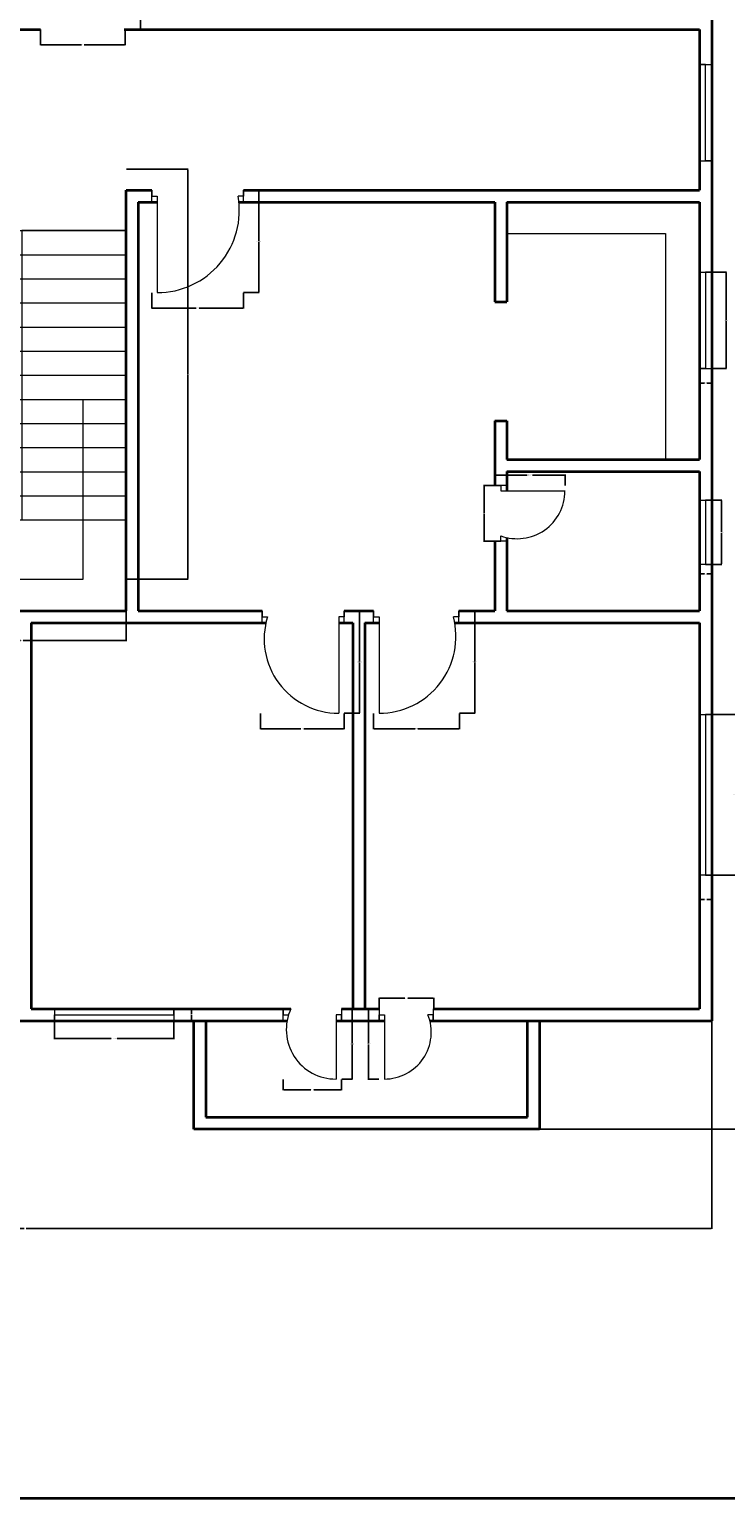
# Model space of a CAD drawing. Units: inches. Extents: x 1944 to 3454, y 1352 to 3055.
# Tile 11 of 17: x 2903 to 3163, y 1352 to 1900. Entities that reach past the tile are written whole.
import ezdxf

# ---------------------------------------------------------------- set-up
doc = ezdxf.new("R2010")
doc.units = ezdxf.units.IN
for name, color, linetype, lineweight in [('A-ANNO-DIMS', 2, 'Continuous', 18), ('A-ANNO-TTLB', 7, 'Continuous', 35), ('A-DOOR', 3, 'Continuous', 20), ('A-FLOR-CASE', 8, 'Continuous', 20), ('A-FLOR-STRS', 7, 'Continuous', 20), ('A-GLAZ', 4, 'Continuous', 18), ('A-WALL', 7, 'Continuous', 35)]:
    doc.layers.add(name, color=color, linetype=linetype, lineweight=lineweight)
doc.styles.get("Standard").update_dxf_attribs({"font": 'arial.ttf'})
doc.dimstyles.get("Standard").update_dxf_attribs({"dimtxt": 0.18, "dimasz": 0.18, "dimexe": 0.18, "dimexo": 0.0625, "dimgap": 0.09, "dimtad": 0, "dimtih": 1, "dimtoh": 1, "dimdec": 4, "dimzin": 0, "dimdsep": 46, "dimtxsty": 'Standard', "dimcen": 0.09, "dimadec": 0, "dimazin": 0, "dimtfac": 1, "dimtdec": 4, "dimtofl": 0, "dimtmove": 0, "dimatfit": 3, "dimfxl": 1, "dimtolj": 1, "dimtzin": 0, "dimarcsym": 0})

# ---------------------------------------------------------------- blocks, each defined once
blk = doc.blocks.new('DOOR-SWING-24IN-07')
for p, q in [((4.5, 20.75), (0, 20.75)), ((0, 20.75), (2.25, 20.75)), ((2.25, 20.75), (2.25, 18.75)), ((2.25, 18.75), (26.25, 18.75)), ((4.5, 0), (0, 0)), ((0, 0), (2.25, 0)), ((2.25, 0), (2.25, 2))]:
    blk.add_line(p, q)
blk.add_arc((8.4, 18.75), 17.84, 249.8228, 0)
blk = doc.blocks.new('DOOR-SWING-36IN-05')
for p, q in [((0, 33.75), (0, 38.25)), ((0, 38.25), (0, 36)), ((0, 36), (0, 36)), ((0, 36), (2, 36)), ((2, 36), (2, 0)), ((31.76, 36), (29.76, 36)), ((31.76, 33.75), (31.76, 38.25)), ((31.76, 38.25), (31.76, 36))]:
    blk.add_line(p, q)
blk.add_arc((2, 28.7), 28.7, 270, 14.7288)
blk = doc.blocks.new('DOOR-SWING-36IN-06')
for p, q in [((0, 33.75), (0, 38.25)), ((0, 38.25), (0, 36)), ((0, 36), (2, 36)), ((30.6, 36), (28.6, 36)), ((28.6, 36), (28.6, 0)), ((30.6, 33.75), (30.6, 38.25)), ((30.6, 38.25), (30.6, 36))]:
    blk.add_line(p, q)
blk.add_arc((28.6, 27.83), 27.83, 162.9212, 270)
blk = doc.blocks.new('DOOR-SWING-24IN-11')
for p, q in [((0, 21.75), (0, 26.25)), ((0, 26.25), (0, 24)), ((0, 24), (2, 24)), ((21.74, 24), (19.74, 24)), ((19.74, 24), (19.74, 0)), ((21.74, 26.25), (21.74, 21.75)), ((21.74, 21.75), (21.74, 24))]:
    blk.add_line(p, q)
blk.add_arc((19.54, 18.41), 18.41, 154.7737, 270.6503)
blk = doc.blocks.new('DOOR-SWING-24IN-12')
for p, q in [((0, 26.25), (0, 21.75)), ((0, 21.75), (0, 24)), ((0, 24), (2, 24)), ((2, 24), (2, 0)), ((20.24, 24), (18.24, 24)), ((20.24, 26.25), (20.24, 21.75)), ((20.24, 21.75), (20.24, 24))]:
    blk.add_line(p, q)
blk.add_arc((2.03, 17.47), 17.47, 269.8982, 21.9448)
blk = doc.blocks.new('DOOR-SWING-36IN-12')
for p, q in [((0, 33.75), (0, 38.25)), ((0, 38.25), (0, 36)), ((0, 36), (2, 36)), ((2, 36), (2, 0)), ((34.2, 36), (32.2, 36)), ((34.2, 33.75), (34.2, 38.25)), ((34.2, 38.25), (34.2, 36))]:
    blk.add_line(p, q)
blk.add_arc((2, 30.67), 30.67, 270, 10.0117)
blk = doc.blocks.new('WINDOW-PLAN-60.00IN-01')
for p, q in [((0, 60), (4.5, 60)), ((4.5, 60), (2.25, 60)), ((2.25, 60), (2.25, 0)), ((4.5, 0), (0, 0)), ((2.25, 0), (4.5, 0))]:
    blk.add_line(p, q)
blk = doc.blocks.new('WINDOW-PLAN-36.00IN-01')
for p, q in [((0, 36), (4.5, 36)), ((4.5, 36), (2.25, 36)), ((2.25, 36), (2.25, 0)), ((2.25, 0), (0, 0)), ((0, 0), (4.5, 0))]:
    blk.add_line(p, q)
blk = doc.blocks.new('WINDOW-PLAN-24.00IN-02')
for p, q in [((0, 24), (4.5, 24)), ((4.5, 24), (2.25, 24)), ((2.25, 24), (2.25, 0)), ((4.5, 0), (0, 0)), ((2.25, 0), (4.5, 0))]:
    blk.add_line(p, q)
blk = doc.blocks.new('WINDOW-PLAN-44.51IN-01')
for p, q in [((0, 4.5), (0, 0)), ((0, 0), (0, 2.25)), ((0, 2.25), (44.51, 2.25)), ((44.51, 2.25), (44.51, 4.5)), ((44.51, 4.5), (44.51, 0))]:
    blk.add_line(p, q)
blk = doc.blocks.new('STAIR-TWO-FLIGHT-01')
for p, q in [((18.12, 152.99), (18.12, 0)), ((0, 130.08), (78, 130.08)), ((78, 130.08), (39, 130.08)), ((39, 130.08), (39, 22.08)), ((0, 121.08), (78, 121.08)), ((0, 112.08), (78, 112.08)), ((0, 103.08), (78, 103.08)), ((0, 94.08), (78, 94.08)), ((0, 85.08), (78, 85.08)), ((0, 76.08), (78, 76.08)), ((0, 67.08), (78, 67.08)), ((61.93, 0), (61.93, 67.08)), ((0, 58.08), (78, 58.08)), ((0, 49.08), (78, 49.08)), ((0, 40.08), (78, 40.08)), ((0, 31.08), (78, 31.08)), ((0, 22.08), (78, 22.08)), ((18.12, 0), (61.93, 0))]:
    blk.add_line(p, q)
blk = doc.blocks.new('*D70')
at = {"layer": 'A-ANNO-DIMS', "color": 0, "lineweight": -2, "transparency": 16777216}
for p, q in [((3157.44, 1809.51), (3162.96, 1809.51)), ((3162.78, 1809.33), (3162.78, 1791.69)), ((3162.78, 1773.69), (3162.78, 1791.32)), ((3157.44, 1773.51), (3162.96, 1773.51))]:
    blk.add_line(p, q, dxfattribs=at)
at = {"layer": 'A-ANNO-DIMS', "color": 0, "transparency": 16777216}
for points in [[(3162.75, 1809.33), (3162.81, 1809.33), (3162.78, 1809.51)], [(3162.75, 1773.69), (3162.81, 1773.69), (3162.78, 1773.51)]]:
    blk.add_solid(points, dxfattribs=at)
at = {"layer": 'Defpoints', "color": 0, "transparency": 16777216}
for p in [(3157.38, 1809.51), (3162.78, 1809.51), (3157.38, 1773.51)]:
    blk.add_point(p, dxfattribs=at)
at = {"layer": 'A-ANNO-DIMS', "color": 0, "transparency": 16777216, "insert": (3162.78, 1791.51), "char_height": 0.18, "attachment_point": 5}
blk.add_mtext('\\A1;WINDOW 36 TYP.', dxfattribs=at)
blk = doc.blocks.new('*D71')
at = {"layer": 'A-ANNO-DIMS', "color": 0, "lineweight": -2, "transparency": 16777216}
for p, q in [((3152.88, 1773.44), (3152.88, 1767.93)), ((3157.38, 1773.44), (3157.38, 1767.93)), ((3153.06, 1768.11), (3154.67, 1768.11)), ((3157.2, 1768.11), (3155.58, 1768.11))]:
    blk.add_line(p, q, dxfattribs=at)
at = {"layer": 'A-ANNO-DIMS', "color": 0, "transparency": 16777216}
for points in [[(3153.06, 1768.14), (3153.06, 1768.08), (3152.88, 1768.11)], [(3157.2, 1768.14), (3157.2, 1768.08), (3157.38, 1768.11)]]:
    blk.add_solid(points, dxfattribs=at)
at = {"layer": 'Defpoints', "color": 0, "transparency": 16777216}
for p in [(3152.88, 1773.51), (3157.38, 1773.51), (3157.38, 1768.11)]:
    blk.add_point(p, dxfattribs=at)
at = {"layer": 'A-ANNO-DIMS', "color": 0, "transparency": 16777216, "insert": (3155.13, 1768.11), "char_height": 0.18, "attachment_point": 5}
blk.add_mtext('\\A1;5 TYP.', dxfattribs=at)
blk = doc.blocks.new('*D76')
at = {"layer": 'A-ANNO-DIMS', "color": 0, "lineweight": -2, "transparency": 16777216}
for p, q in [((3157.44, 1724.44), (3161.16, 1724.44)), ((3160.98, 1724.26), (3160.98, 1712.63)), ((3160.98, 1700.62), (3160.98, 1712.26)), ((3157.44, 1700.44), (3161.16, 1700.44))]:
    blk.add_line(p, q, dxfattribs=at)
at = {"layer": 'A-ANNO-DIMS', "color": 0, "transparency": 16777216}
for points in [[(3160.95, 1724.26), (3161.01, 1724.26), (3160.98, 1724.44)], [(3160.95, 1700.62), (3161.01, 1700.62), (3160.98, 1700.44)]]:
    blk.add_solid(points, dxfattribs=at)
at = {"layer": 'Defpoints', "color": 0, "transparency": 16777216}
for p in [(3157.38, 1724.44), (3160.98, 1724.44), (3157.38, 1700.44)]:
    blk.add_point(p, dxfattribs=at)
at = {"layer": 'A-ANNO-DIMS', "color": 0, "transparency": 16777216, "insert": (3160.98, 1712.44), "char_height": 0.18, "attachment_point": 5}
blk.add_mtext('\\A1;WINDOW 24 TYP.', dxfattribs=at)
blk = doc.blocks.new('*D77')
at = {"layer": 'A-ANNO-DIMS', "color": 0, "lineweight": -2, "transparency": 16777216}
for p, q in [((3152.88, 1700.38), (3152.88, 1696.66)), ((3157.38, 1700.38), (3157.38, 1696.66)), ((3153.06, 1696.84), (3154.67, 1696.84)), ((3157.2, 1696.84), (3155.58, 1696.84))]:
    blk.add_line(p, q, dxfattribs=at)
at = {"layer": 'A-ANNO-DIMS', "color": 0, "transparency": 16777216}
for points in [[(3153.06, 1696.87), (3153.06, 1696.81), (3152.88, 1696.84)], [(3157.2, 1696.87), (3157.2, 1696.81), (3157.38, 1696.84)]]:
    blk.add_solid(points, dxfattribs=at)
at = {"layer": 'Defpoints', "color": 0, "transparency": 16777216}
for p in [(3152.88, 1700.44), (3157.38, 1700.44), (3157.38, 1696.84)]:
    blk.add_point(p, dxfattribs=at)
at = {"layer": 'A-ANNO-DIMS', "color": 0, "transparency": 16777216, "insert": (3155.13, 1696.84), "char_height": 0.18, "attachment_point": 5}
blk.add_mtext('\\A1;5 TYP.', dxfattribs=at)
blk = doc.blocks.new('*D78')
at = {"layer": 'A-ANNO-DIMS', "color": 0, "lineweight": -2, "transparency": 16777216}
for p, q in [((3157.44, 1644.39), (3166.56, 1644.39)), ((3166.38, 1644.21), (3166.38, 1614.57)), ((3166.38, 1584.57), (3166.38, 1614.21)), ((3157.44, 1584.39), (3166.56, 1584.39))]:
    blk.add_line(p, q, dxfattribs=at)
at = {"layer": 'A-ANNO-DIMS', "color": 0, "transparency": 16777216}
for points in [[(3166.35, 1644.21), (3166.41, 1644.21), (3166.38, 1644.39)], [(3166.35, 1584.57), (3166.41, 1584.57), (3166.38, 1584.39)]]:
    blk.add_solid(points, dxfattribs=at)
at = {"layer": 'Defpoints', "color": 0, "transparency": 16777216}
for p in [(3157.38, 1644.39), (3166.38, 1644.39), (3157.38, 1584.39)]:
    blk.add_point(p, dxfattribs=at)
at = {"layer": 'A-ANNO-DIMS', "color": 0, "transparency": 16777216, "insert": (3166.38, 1614.39), "char_height": 0.18, "attachment_point": 5}
blk.add_mtext('\\A1;WINDOW 60 TYP.', dxfattribs=at)
blk = doc.blocks.new('*D79')
at = {"layer": 'A-ANNO-DIMS', "color": 0, "lineweight": -2, "transparency": 16777216}
for p, q in [((3152.88, 1584.33), (3152.88, 1575.21)), ((3157.38, 1584.33), (3157.38, 1575.21)), ((3153.06, 1575.39), (3154.67, 1575.39)), ((3157.2, 1575.39), (3155.58, 1575.39))]:
    blk.add_line(p, q, dxfattribs=at)
at = {"layer": 'A-ANNO-DIMS', "color": 0, "transparency": 16777216}
for points in [[(3153.06, 1575.42), (3153.06, 1575.36), (3152.88, 1575.39)], [(3157.2, 1575.42), (3157.2, 1575.36), (3157.38, 1575.39)]]:
    blk.add_solid(points, dxfattribs=at)
at = {"layer": 'Defpoints', "color": 0, "transparency": 16777216}
for p in [(3152.88, 1584.39), (3157.38, 1584.39), (3157.38, 1575.39)]:
    blk.add_point(p, dxfattribs=at)
at = {"layer": 'A-ANNO-DIMS', "color": 0, "transparency": 16777216, "insert": (3155.13, 1575.39), "char_height": 0.18, "attachment_point": 5}
blk.add_mtext('\\A1;5 TYP.', dxfattribs=at)
blk = doc.blocks.new('*D82')
at = {"layer": 'A-ANNO-DIMS', "color": 0, "lineweight": -2, "transparency": 16777216}
for p, q in [((2912.07, 1530.03), (2912.07, 1523.24)), ((2956.59, 1530.03), (2956.59, 1523.24)), ((2912.25, 1523.42), (2933.21, 1523.42)), ((2956.41, 1523.42), (2935.45, 1523.42))]:
    blk.add_line(p, q, dxfattribs=at)
at = {"layer": 'A-ANNO-DIMS', "color": 0, "transparency": 16777216}
for points in [[(2912.25, 1523.45), (2912.25, 1523.39), (2912.07, 1523.42)], [(2956.41, 1523.45), (2956.41, 1523.39), (2956.59, 1523.42)]]:
    blk.add_solid(points, dxfattribs=at)
at = {"layer": 'Defpoints', "color": 0, "transparency": 16777216}
for p in [(2912.07, 1530.1), (2956.59, 1530.1), (2956.59, 1523.42)]:
    blk.add_point(p, dxfattribs=at)
at = {"layer": 'A-ANNO-DIMS', "color": 0, "transparency": 16777216, "insert": (2934.33, 1523.42), "char_height": 0.18, "attachment_point": 5}
blk.add_mtext('\\A1;WINDOW 45 TYP.', dxfattribs=at)
blk = doc.blocks.new('*D83')
at = {"layer": 'A-ANNO-DIMS', "color": 0, "lineweight": -2, "transparency": 16777216}
for p, q in [((2956.65, 1534.6), (2963.44, 1534.6)), ((2956.65, 1530.1), (2963.44, 1530.1)), ((2963.26, 1534.42), (2963.26, 1532.53)), ((2963.26, 1530.28), (2963.26, 1532.16))]:
    blk.add_line(p, q, dxfattribs=at)
at = {"layer": 'A-ANNO-DIMS', "color": 0, "transparency": 16777216}
for points in [[(2963.23, 1534.42), (2963.29, 1534.42), (2963.26, 1534.6)], [(2963.23, 1530.28), (2963.29, 1530.28), (2963.26, 1530.1)]]:
    blk.add_solid(points, dxfattribs=at)
at = {"layer": 'Defpoints', "color": 0, "transparency": 16777216}
for p in [(2956.59, 1534.6), (2956.59, 1530.1), (2963.26, 1534.6)]:
    blk.add_point(p, dxfattribs=at)
at = {"layer": 'A-ANNO-DIMS', "color": 0, "transparency": 16777216, "insert": (2963.26, 1532.35), "char_height": 0.18, "attachment_point": 5}
blk.add_mtext('\\A1;5 TYP.', dxfattribs=at)
blk = doc.blocks.new('*D90')
at = {"layer": 'A-ANNO-DIMS', "color": 0, "lineweight": -2, "transparency": 16777216}
for p, q in [((2938.94, 1847.92), (2962, 1847.92)), ((2961.82, 1847.74), (2961.82, 1771.6)), ((2961.82, 1695.1), (2961.82, 1771.24)), ((2938.94, 1694.92), (2962, 1694.92))]:
    blk.add_line(p, q, dxfattribs=at)
at = {"layer": 'A-ANNO-DIMS', "color": 0, "transparency": 16777216}
for points in [[(2961.79, 1847.74), (2961.85, 1847.74), (2961.82, 1847.92)], [(2961.79, 1695.1), (2961.85, 1695.1), (2961.82, 1694.92)]]:
    blk.add_solid(points, dxfattribs=at)
at = {"layer": 'Defpoints', "color": 0, "transparency": 16777216}
for p in [(2938.88, 1847.92), (2961.82, 1847.92), (2938.88, 1694.92)]:
    blk.add_point(p, dxfattribs=at)
at = {"layer": 'A-ANNO-DIMS', "color": 0, "transparency": 16777216, "insert": (2961.82, 1771.42), "char_height": 0.18, "attachment_point": 5}
blk.add_mtext('\\A1;STAIR 153 TYP.', dxfattribs=at)
blk = doc.blocks.new('*D91')
at = {"layer": 'A-ANNO-DIMS', "color": 0, "lineweight": -2, "transparency": 16777216}
for p, q in [((2860.88, 1694.86), (2860.88, 1671.8)), ((2938.88, 1694.86), (2938.88, 1671.8)), ((2861.06, 1671.98), (2899.35, 1671.98)), ((2938.7, 1671.98), (2900.4, 1671.98))]:
    blk.add_line(p, q, dxfattribs=at)
at = {"layer": 'A-ANNO-DIMS', "color": 0, "transparency": 16777216}
for points in [[(2861.06, 1672.01), (2861.06, 1671.95), (2860.88, 1671.98)], [(2938.7, 1672.01), (2938.7, 1671.95), (2938.88, 1671.98)]]:
    blk.add_solid(points, dxfattribs=at)
at = {"layer": 'Defpoints', "color": 0, "transparency": 16777216}
for p in [(2860.88, 1694.92), (2938.88, 1694.92), (2938.88, 1671.98)]:
    blk.add_point(p, dxfattribs=at)
at = {"layer": 'A-ANNO-DIMS', "color": 0, "transparency": 16777216, "insert": (2899.88, 1671.98), "char_height": 0.18, "attachment_point": 5}
blk.add_mtext('\\A1;78 TYP.', dxfattribs=at)
blk = doc.blocks.new('*D100')
at = {"layer": 'A-ANNO-DIMS', "color": 0, "lineweight": -2, "transparency": 16777216}
for p, q in [((3063.29, 1683.1), (3069.15, 1683.1)), ((3068.97, 1682.92), (3068.97, 1664.15)), ((3068.97, 1645.03), (3068.97, 1663.79)), ((3063.29, 1644.85), (3069.15, 1644.85))]:
    blk.add_line(p, q, dxfattribs=at)
at = {"layer": 'A-ANNO-DIMS', "color": 0, "transparency": 16777216}
for points in [[(3068.94, 1682.92), (3069, 1682.92), (3068.97, 1683.1)], [(3068.94, 1645.03), (3069, 1645.03), (3068.97, 1644.85)]]:
    blk.add_solid(points, dxfattribs=at)
at = {"layer": 'Defpoints', "color": 0, "transparency": 16777216}
for p in [(3063.23, 1683.1), (3068.97, 1683.1), (3063.23, 1644.85)]:
    blk.add_point(p, dxfattribs=at)
at = {"layer": 'A-ANNO-DIMS', "color": 0, "transparency": 16777216, "insert": (3068.97, 1663.97), "char_height": 0.18, "attachment_point": 5}
blk.add_mtext('\\A1;SWING 38 TYP.', dxfattribs=at)
blk = doc.blocks.new('*D101')
at = {"layer": 'A-ANNO-DIMS', "color": 0, "lineweight": -2, "transparency": 16777216}
for p, q in [((3031.21, 1644.78), (3031.21, 1638.93)), ((3063.23, 1644.78), (3063.23, 1638.93)), ((3031.39, 1639.11), (3046.69, 1639.11)), ((3063.05, 1639.11), (3047.75, 1639.11))]:
    blk.add_line(p, q, dxfattribs=at)
at = {"layer": 'A-ANNO-DIMS', "color": 0, "transparency": 16777216}
for points in [[(3031.39, 1639.14), (3031.39, 1639.08), (3031.21, 1639.11)], [(3063.05, 1639.14), (3063.05, 1639.08), (3063.23, 1639.11)]]:
    blk.add_solid(points, dxfattribs=at)
at = {"layer": 'Defpoints', "color": 0, "transparency": 16777216}
for p in [(3031.21, 1644.85), (3063.23, 1644.85), (3063.23, 1639.11)]:
    blk.add_point(p, dxfattribs=at)
at = {"layer": 'A-ANNO-DIMS', "color": 0, "transparency": 16777216, "insert": (3047.22, 1639.11), "char_height": 0.18, "attachment_point": 5}
blk.add_mtext('\\A1;32 TYP.', dxfattribs=at)
blk = doc.blocks.new('*D102')
at = {"layer": 'A-ANNO-DIMS', "color": 0, "lineweight": -2, "transparency": 16777216}
for p, q in [((3020.23, 1683.1), (3026.09, 1683.1)), ((3025.91, 1682.92), (3025.91, 1664.15)), ((3025.91, 1645.03), (3025.91, 1663.79)), ((3020.23, 1644.85), (3026.09, 1644.85))]:
    blk.add_line(p, q, dxfattribs=at)
at = {"layer": 'A-ANNO-DIMS', "color": 0, "transparency": 16777216}
for points in [[(3025.88, 1682.92), (3025.94, 1682.92), (3025.91, 1683.1)], [(3025.88, 1645.03), (3025.94, 1645.03), (3025.91, 1644.85)]]:
    blk.add_solid(points, dxfattribs=at)
at = {"layer": 'Defpoints', "color": 0, "transparency": 16777216}
for p in [(3020.17, 1683.1), (3025.91, 1683.1), (3020.17, 1644.85)]:
    blk.add_point(p, dxfattribs=at)
at = {"layer": 'A-ANNO-DIMS', "color": 0, "transparency": 16777216, "insert": (3025.91, 1663.97), "char_height": 0.18, "attachment_point": 5}
blk.add_mtext('\\A1;SWING 38 TYP.', dxfattribs=at)
blk = doc.blocks.new('*D103')
at = {"layer": 'A-ANNO-DIMS', "color": 0, "lineweight": -2, "transparency": 16777216}
for p, q in [((2988.97, 1644.78), (2988.97, 1638.93)), ((3020.17, 1644.78), (3020.17, 1638.93)), ((2989.15, 1639.11), (3004.04, 1639.11)), ((3019.99, 1639.11), (3005.1, 1639.11))]:
    blk.add_line(p, q, dxfattribs=at)
at = {"layer": 'A-ANNO-DIMS', "color": 0, "transparency": 16777216}
for points in [[(2989.15, 1639.14), (2989.15, 1639.08), (2988.97, 1639.11)], [(3019.99, 1639.14), (3019.99, 1639.08), (3020.17, 1639.11)]]:
    blk.add_solid(points, dxfattribs=at)
at = {"layer": 'Defpoints', "color": 0, "transparency": 16777216}
for p in [(2988.97, 1644.85), (3020.17, 1644.85), (3020.17, 1639.11)]:
    blk.add_point(p, dxfattribs=at)
at = {"layer": 'A-ANNO-DIMS', "color": 0, "transparency": 16777216, "insert": (3004.57, 1639.11), "char_height": 0.18, "attachment_point": 5}
blk.add_mtext('\\A1;31 TYP.', dxfattribs=at)
blk = doc.blocks.new('*D108')
at = {"layer": 'A-ANNO-DIMS', "color": 0, "lineweight": -2, "transparency": 16777216}
for p, q in [((2938.5, 1938.35), (2944.35, 1938.35)), ((2944.17, 1938.17), (2944.17, 1919.4)), ((2944.17, 1900.28), (2944.17, 1919.04)), ((2938.5, 1900.1), (2944.35, 1900.1))]:
    blk.add_line(p, q, dxfattribs=at)
at = {"layer": 'A-ANNO-DIMS', "color": 0, "transparency": 16777216}
for points in [[(2944.14, 1938.17), (2944.2, 1938.17), (2944.17, 1938.35)], [(2944.14, 1900.28), (2944.2, 1900.28), (2944.17, 1900.1)]]:
    blk.add_solid(points, dxfattribs=at)
at = {"layer": 'Defpoints', "color": 0, "transparency": 16777216}
for p in [(2938.44, 1938.35), (2944.17, 1938.35), (2938.44, 1900.1)]:
    blk.add_point(p, dxfattribs=at)
at = {"layer": 'A-ANNO-DIMS', "color": 0, "transparency": 16777216, "insert": (2944.17, 1919.22), "char_height": 0.18, "attachment_point": 5}
blk.add_mtext('\\A1;SWING 38 TYP.', dxfattribs=at)
blk = doc.blocks.new('*D109')
at = {"layer": 'A-ANNO-DIMS', "color": 0, "lineweight": -2, "transparency": 16777216}
for p, q in [((2906.83, 1900.03), (2906.83, 1894.18)), ((2938.44, 1900.03), (2938.44, 1894.18)), ((2907.01, 1894.36), (2922.11, 1894.36)), ((2938.26, 1894.36), (2923.16, 1894.36))]:
    blk.add_line(p, q, dxfattribs=at)
at = {"layer": 'A-ANNO-DIMS', "color": 0, "transparency": 16777216}
for points in [[(2907.01, 1894.39), (2907.01, 1894.33), (2906.83, 1894.36)], [(2938.26, 1894.39), (2938.26, 1894.33), (2938.44, 1894.36)]]:
    blk.add_solid(points, dxfattribs=at)
at = {"layer": 'Defpoints', "color": 0, "transparency": 16777216}
for p in [(2906.83, 1900.1), (2938.44, 1900.1), (2938.44, 1894.36)]:
    blk.add_point(p, dxfattribs=at)
at = {"layer": 'A-ANNO-DIMS', "color": 0, "transparency": 16777216, "insert": (2922.63, 1894.36), "char_height": 0.18, "attachment_point": 5}
blk.add_mtext('\\A1;32 TYP.', dxfattribs=at)
blk = doc.blocks.new('*D114')
at = {"layer": 'A-ANNO-DIMS', "color": 0, "lineweight": -2, "transparency": 16777216}
for p, q in [((2982.66, 1840.1), (2988.51, 1840.1)), ((2988.33, 1839.92), (2988.33, 1821.15)), ((2988.33, 1802.03), (2988.33, 1820.79)), ((2982.66, 1801.85), (2988.51, 1801.85))]:
    blk.add_line(p, q, dxfattribs=at)
at = {"layer": 'A-ANNO-DIMS', "color": 0, "transparency": 16777216}
for points in [[(2988.3, 1839.92), (2988.36, 1839.92), (2988.33, 1840.1)], [(2988.3, 1802.03), (2988.36, 1802.03), (2988.33, 1801.85)]]:
    blk.add_solid(points, dxfattribs=at)
at = {"layer": 'Defpoints', "color": 0, "transparency": 16777216}
for p in [(2982.59, 1840.1), (2988.33, 1840.1), (2982.59, 1801.85)]:
    blk.add_point(p, dxfattribs=at)
at = {"layer": 'A-ANNO-DIMS', "color": 0, "transparency": 16777216, "insert": (2988.33, 1820.97), "char_height": 0.18, "attachment_point": 5}
blk.add_mtext('\\A1;SWING 38 TYP.', dxfattribs=at)
blk = doc.blocks.new('*D115')
at = {"layer": 'A-ANNO-DIMS', "color": 0, "lineweight": -2, "transparency": 16777216}
for p, q in [((2948.39, 1801.78), (2948.39, 1795.93)), ((2982.59, 1801.78), (2982.59, 1795.93)), ((2948.57, 1796.11), (2964.96, 1796.11)), ((2982.41, 1796.11), (2966.02, 1796.11))]:
    blk.add_line(p, q, dxfattribs=at)
at = {"layer": 'A-ANNO-DIMS', "color": 0, "transparency": 16777216}
for points in [[(2948.57, 1796.14), (2948.57, 1796.08), (2948.39, 1796.11)], [(2982.41, 1796.14), (2982.41, 1796.08), (2982.59, 1796.11)]]:
    blk.add_solid(points, dxfattribs=at)
at = {"layer": 'Defpoints', "color": 0, "transparency": 16777216}
for p in [(2948.39, 1801.85), (2982.59, 1801.85), (2982.59, 1796.11)]:
    blk.add_point(p, dxfattribs=at)
at = {"layer": 'A-ANNO-DIMS', "color": 0, "transparency": 16777216, "insert": (2965.49, 1796.11), "char_height": 0.18, "attachment_point": 5}
blk.add_mtext('\\A1;34 TYP.', dxfattribs=at)
blk = doc.blocks.new('*D128')
at = {"layer": 'A-ANNO-DIMS', "color": 0, "lineweight": -2, "transparency": 16777216}
for p, q in [((3076.38, 1729.91), (3076.38, 1733.96)), ((3076.56, 1733.78), (3088.51, 1733.78)), ((3102.45, 1733.78), (3090.49, 1733.78)), ((3102.63, 1729.91), (3102.63, 1733.96))]:
    blk.add_line(p, q, dxfattribs=at)
at = {"layer": 'A-ANNO-DIMS', "color": 0, "transparency": 16777216}
for points in [[(3076.56, 1733.81), (3076.56, 1733.75), (3076.38, 1733.78)], [(3102.45, 1733.81), (3102.45, 1733.75), (3102.63, 1733.78)]]:
    blk.add_solid(points, dxfattribs=at)
at = {"layer": 'Defpoints', "color": 0, "transparency": 16777216}
for p in [(3102.63, 1733.78), (3076.38, 1729.85), (3102.63, 1729.85)]:
    blk.add_point(p, dxfattribs=at)
at = {"layer": 'A-ANNO-DIMS', "color": 0, "transparency": 16777216, "insert": (3089.5, 1733.78), "char_height": 0.18, "attachment_point": 5}
blk.add_mtext('\\A1;SWING 26 TYP.', dxfattribs=at)
blk = doc.blocks.new('*D129')
at = {"layer": 'A-ANNO-DIMS', "color": 0, "lineweight": -2, "transparency": 16777216}
for p, q in [((3076.31, 1729.85), (3072.26, 1729.85)), ((3072.44, 1729.67), (3072.44, 1719.65)), ((3072.44, 1709.26), (3072.44, 1719.29)), ((3076.31, 1709.08), (3072.26, 1709.08))]:
    blk.add_line(p, q, dxfattribs=at)
at = {"layer": 'A-ANNO-DIMS', "color": 0, "transparency": 16777216}
for points in [[(3072.41, 1729.67), (3072.47, 1729.67), (3072.44, 1729.85)], [(3072.41, 1709.26), (3072.47, 1709.26), (3072.44, 1709.08)]]:
    blk.add_solid(points, dxfattribs=at)
at = {"layer": 'Defpoints', "color": 0, "transparency": 16777216}
for p in [(3072.44, 1729.85), (3076.38, 1729.85), (3076.38, 1709.08)]:
    blk.add_point(p, dxfattribs=at)
at = {"layer": 'A-ANNO-DIMS', "color": 0, "transparency": 16777216, "insert": (3072.44, 1719.47), "char_height": 0.18, "attachment_point": 5}
blk.add_mtext('\\A1;21 TYP.', dxfattribs=at)
blk = doc.blocks.new('*D136')
at = {"layer": 'A-ANNO-DIMS', "color": 0, "lineweight": -2, "transparency": 16777216}
for p, q in [((3019.27, 1534.6), (3023.34, 1534.6)), ((3023.16, 1534.42), (3023.16, 1521.62)), ((3023.16, 1508.45), (3023.16, 1521.25)), ((3019.27, 1508.27), (3023.34, 1508.27))]:
    blk.add_line(p, q, dxfattribs=at)
at = {"layer": 'A-ANNO-DIMS', "color": 0, "transparency": 16777216}
for points in [[(3023.13, 1534.42), (3023.19, 1534.42), (3023.16, 1534.6)], [(3023.13, 1508.45), (3023.19, 1508.45), (3023.16, 1508.27)]]:
    blk.add_solid(points, dxfattribs=at)
at = {"layer": 'Defpoints', "color": 0, "transparency": 16777216}
for p in [(3019.21, 1534.6), (3023.16, 1534.6), (3019.21, 1508.27)]:
    blk.add_point(p, dxfattribs=at)
at = {"layer": 'A-ANNO-DIMS', "color": 0, "transparency": 16777216, "insert": (3023.16, 1521.44), "char_height": 0.18, "attachment_point": 5}
blk.add_mtext('\\A1;SWING 26 TYP.', dxfattribs=at)
blk = doc.blocks.new('*D137')
at = {"layer": 'A-ANNO-DIMS', "color": 0, "lineweight": -2, "transparency": 16777216}
for p, q in [((2997.47, 1508.21), (2997.47, 1504.15)), ((3019.21, 1508.21), (3019.21, 1504.15)), ((2997.65, 1504.33), (3007.81, 1504.33)), ((3019.03, 1504.33), (3008.87, 1504.33))]:
    blk.add_line(p, q, dxfattribs=at)
at = {"layer": 'A-ANNO-DIMS', "color": 0, "transparency": 16777216}
for points in [[(2997.65, 1504.36), (2997.65, 1504.3), (2997.47, 1504.33)], [(3019.03, 1504.36), (3019.03, 1504.3), (3019.21, 1504.33)]]:
    blk.add_solid(points, dxfattribs=at)
at = {"layer": 'Defpoints', "color": 0, "transparency": 16777216}
for p in [(2997.47, 1508.27), (3019.21, 1508.27), (3019.21, 1504.33)]:
    blk.add_point(p, dxfattribs=at)
at = {"layer": 'A-ANNO-DIMS', "color": 0, "transparency": 16777216, "insert": (3008.34, 1504.33), "char_height": 0.18, "attachment_point": 5}
blk.add_mtext('\\A1;22 TYP.', dxfattribs=at)
blk = doc.blocks.new('*D138')
at = {"layer": 'A-ANNO-DIMS', "color": 0, "lineweight": -2, "transparency": 16777216}
for p, q in [((3033.15, 1534.6), (3029.09, 1534.6)), ((3029.27, 1534.42), (3029.27, 1521.65)), ((3029.27, 1508.52), (3029.27, 1521.28)), ((3033.15, 1508.34), (3029.09, 1508.34))]:
    blk.add_line(p, q, dxfattribs=at)
at = {"layer": 'A-ANNO-DIMS', "color": 0, "transparency": 16777216}
for points in [[(3029.24, 1534.42), (3029.3, 1534.42), (3029.27, 1534.6)], [(3029.24, 1508.52), (3029.3, 1508.52), (3029.27, 1508.34)]]:
    blk.add_solid(points, dxfattribs=at)
at = {"layer": 'Defpoints', "color": 0, "transparency": 16777216}
for p in [(3029.27, 1534.6), (3033.21, 1534.6), (3033.21, 1508.34)]:
    blk.add_point(p, dxfattribs=at)
at = {"layer": 'A-ANNO-DIMS', "color": 0, "transparency": 16777216, "insert": (3029.27, 1521.47), "char_height": 0.18, "attachment_point": 5}
blk.add_mtext('\\A1;SWING 26 TYP.', dxfattribs=at)
blk = doc.blocks.new('*D139')
at = {"layer": 'A-ANNO-DIMS', "color": 0, "lineweight": -2, "transparency": 16777216}
for p, q in [((3033.21, 1534.66), (3033.21, 1538.72)), ((3033.39, 1538.54), (3042.88, 1538.54)), ((3053.44, 1538.54), (3043.94, 1538.54)), ((3053.62, 1534.66), (3053.62, 1538.72))]:
    blk.add_line(p, q, dxfattribs=at)
at = {"layer": 'A-ANNO-DIMS', "color": 0, "transparency": 16777216}
for points in [[(3033.39, 1538.57), (3033.39, 1538.51), (3033.21, 1538.54)], [(3053.44, 1538.57), (3053.44, 1538.51), (3053.62, 1538.54)]]:
    blk.add_solid(points, dxfattribs=at)
at = {"layer": 'Defpoints', "color": 0, "transparency": 16777216}
for p in [(3053.62, 1538.54), (3033.21, 1534.6), (3053.62, 1534.6)]:
    blk.add_point(p, dxfattribs=at)
at = {"layer": 'A-ANNO-DIMS', "color": 0, "transparency": 16777216, "insert": (3043.41, 1538.54), "char_height": 0.18, "attachment_point": 5}
blk.add_mtext('\\A1;20 TYP.', dxfattribs=at)
blk = doc.blocks.new('*D186')
at = {"layer": 'A-ANNO-DIMS', "color": 0, "lineweight": -2, "transparency": 16777216}
for p, q in [((2644.88, 1530.03), (2644.88, 1452.42)), ((3157.38, 1530.03), (3157.38, 1452.42)), ((2645.06, 1452.6), (2900.73, 1452.6)), ((3157.2, 1452.6), (2901.52, 1452.6))]:
    blk.add_line(p, q, dxfattribs=at)
at = {"layer": 'A-ANNO-DIMS', "color": 0, "transparency": 16777216}
for points in [[(2645.06, 1452.63), (2645.06, 1452.57), (2644.88, 1452.6)], [(3157.2, 1452.63), (3157.2, 1452.57), (3157.38, 1452.6)]]:
    blk.add_solid(points, dxfattribs=at)
at = {"layer": 'Defpoints', "color": 0, "transparency": 16777216}
for p in [(2644.88, 1530.1), (3157.38, 1530.1), (3157.38, 1452.6)]:
    blk.add_point(p, dxfattribs=at)
at = {"layer": 'A-ANNO-DIMS', "color": 0, "transparency": 16777216, "insert": (2901.13, 1452.6), "char_height": 0.18, "attachment_point": 5}
blk.add_mtext('\\A1;512.5', dxfattribs=at)
blk = doc.blocks.new('*D187')
at = {"layer": 'A-ANNO-DIMS', "color": 0, "lineweight": -2, "transparency": 16777216}
for p, q in [((3089.53, 2222.6), (3245.46, 2222.6)), ((3245.28, 2222.42), (3245.28, 1856.28)), ((3245.28, 1489.78), (3245.28, 1855.91)), ((3093.18, 1489.6), (3245.46, 1489.6))]:
    blk.add_line(p, q, dxfattribs=at)
at = {"layer": 'A-ANNO-DIMS', "color": 0, "transparency": 16777216}
for points in [[(3245.25, 2222.42), (3245.31, 2222.42), (3245.28, 2222.6)], [(3245.25, 1489.78), (3245.31, 1489.78), (3245.28, 1489.6)]]:
    blk.add_solid(points, dxfattribs=at)
at = {"layer": 'Defpoints', "color": 0, "transparency": 16777216}
for p in [(3089.47, 2222.6), (3245.28, 2222.6), (3093.12, 1489.6)]:
    blk.add_point(p, dxfattribs=at)
at = {"layer": 'A-ANNO-DIMS', "color": 0, "transparency": 16777216, "insert": (3245.28, 1856.1), "char_height": 0.18, "attachment_point": 5}
blk.add_mtext('\\A1;733', dxfattribs=at)

msp = doc.modelspace()

# ---------------------------------------------------------------- linework, layer by layer
at = {"layer": 'A-ANNO-TTLB'}
msp.add_lwpolyline([(1943.914, 3054.605), (3453.633, 3054.605), (3453.633, 1351.76), (1943.914, 1351.76)], close=True, dxfattribs=at)
at = {"layer": 'A-FLOR-CASE'}
for p, q in [((3080.875, 1823.863), (3140.193, 1823.863)), ((3140.193, 1823.863), (3140.193, 1739.596))]:
    msp.add_line(p, q, dxfattribs=at)
at = {"layer": 'A-WALL'}
for p, q in [((3157.375, 2182.096), (3157.375, 1530.096)), ((2895.494, 1900.096), (2906.831, 1900.096)), ((2938.072, 1900.096), (3064.375, 1900.096)), ((3064.375, 1900.096), (3152.875, 1900.096)), ((3152.875, 1900.096), (3152.875, 1840.096)), ((3152.875, 1900.096), (3152.875, 1895.596)), ((2938.875, 1840.096), (2948.392, 1840.096)), ((2938.875, 1683.096), (2938.875, 1840.096)), ((2982.593, 1840.096), (3152.875, 1840.096)), ((2943.375, 1835.596), (2950.392, 1835.596)), ((2943.375, 1835.596), (2943.375, 1683.096)), ((2980.905, 1835.596), (3076.375, 1835.596)), ((3076.375, 1835.596), (3076.375, 1798.423)), ((3080.875, 1835.596), (3080.875, 1798.423)), ((3080.875, 1835.596), (3152.875, 1835.596)), ((3152.875, 1835.596), (3152.875, 1739.596)), ((3076.375, 1798.423), (3080.875, 1798.423)), ((3076.375, 1754.002), (3076.375, 1729.846)), ((3076.375, 1754.002), (3080.875, 1754.002)), ((3080.875, 1754.002), (3080.875, 1739.596)), ((3080.875, 1739.596), (3152.875, 1739.596)), ((3080.875, 1735.096), (3080.875, 1727.846)), ((3080.875, 1735.096), (3152.875, 1735.096)), ((3152.875, 1735.096), (3152.875, 1683.096)), ((3076.375, 1709.096), (3076.375, 1683.096)), ((3080.875, 1710.434), (3080.875, 1683.096)), ((2860.875, 1683.096), (2938.875, 1683.096)), ((2903.375, 1678.596), (2903.375, 1534.596)), ((2903.375, 1678.596), (2990.978, 1678.596)), ((2943.375, 1683.096), (2989.567, 1683.096)), ((3018.168, 1678.596), (3023.375, 1678.596)), ((3020.168, 1683.096), (3031.21, 1683.096)), ((3023.375, 1678.596), (3023.375, 1534.596)), ((3027.875, 1678.596), (3027.875, 1534.596)), ((3027.875, 1678.596), (3033.21, 1678.596)), ((3061.465, 1678.596), (3076.375, 1678.596)), ((3062.969, 1683.096), (3076.375, 1683.096)), ((3076.375, 1678.596), (3152.875, 1678.596)), ((3080.875, 1683.096), (3152.875, 1683.096)), ((3080.875, 1683.096), (3152.875, 1683.096)), ((3152.875, 1678.596), (3152.875, 1534.596)), ((2804.91, 1530.096), (2998.902, 1530.096)), ((2903.375, 1534.596), (3000.351, 1534.596)), ((2964.12, 1489.596), (2964.12, 1530.096)), ((2968.62, 1530.096), (2968.62, 1494.096)), ((3017.211, 1530.096), (3035.21, 1530.096)), ((3019.211, 1534.596), (3033.21, 1534.596)), ((3052.18, 1530.096), (3157.375, 1530.096)), ((3053.446, 1534.596), (3152.875, 1534.596)), ((3088.62, 1494.096), (3088.62, 1530.096)), ((3088.62, 1530.096), (3093.12, 1530.096)), ((3093.12, 1530.096), (3093.12, 1494.096)), ((2968.62, 1494.096), (3088.62, 1494.096)), ((3093.12, 1494.096), (3093.12, 1489.596)), ((2968.62, 1489.596), (2964.12, 1489.596)), ((3093.12, 1489.596), (2968.62, 1489.596))]:
    msp.add_line(p, q, dxfattribs=at)

# ---------------------------------------------------------------- block references
at = {"layer": 'A-DOOR'}
for name, p in [('DOOR-SWING-36IN-12', (2948.392, 1801.846)), ('DOOR-SWING-24IN-07', (3076.376, 1709.096)), ('DOOR-SWING-36IN-06', (2989.568, 1644.846)), ('DOOR-SWING-36IN-05', (3031.21, 1644.846)), ('DOOR-SWING-24IN-11', (2997.467, 1508.346)), ('DOOR-SWING-24IN-12', (3033.21, 1508.346))]:
    msp.add_blockref(name, p, dxfattribs=at)
at = {"layer": 'A-FLOR-STRS'}
msp.add_blockref('STAIR-TWO-FLIGHT-01', (2860.876, 1694.924), dxfattribs=at)
at = {"layer": 'A-GLAZ', "extrusion": (0, 0, -1), "zscale": -1, "rotation": 180}
msp.add_blockref('WINDOW-PLAN-36.00IN-01', (-3152.876, 1887.047), dxfattribs=at)
at = {"layer": 'A-GLAZ'}
for name, p in [('WINDOW-PLAN-36.00IN-01', (3152.876, 1773.506)), ('WINDOW-PLAN-24.00IN-02', (3152.876, 1700.442)), ('WINDOW-PLAN-60.00IN-01', (3152.876, 1584.389)), ('WINDOW-PLAN-44.51IN-01', (2912.075, 1530.096))]:
    msp.add_blockref(name, p, dxfattribs=at)

# ---------------------------------------------------------------- dimensions: what is measured, and where the dimension line sits
at = {"layer": 'A-ANNO-DIMS'}
dim = msp.add_linear_dim(base=(3245.282, 2222.596), p1=(3093.12, 1489.596), p2=(3089.47, 2222.596), angle=90, dimstyle='Standard', override={"dimdec": 0, "dimlfac": 1, "dimrnd": 0, "dimzin": 0, "dimdsep": 46, "dimlunit": 2}, dxfattribs=at)
dim.commit()
dim.dimension.update_dxf_attribs({"geometry": '*D187', "text_midpoint": (3245.282, 1856.096)})
for base, p1, p2, text, picture, middle in [((2944.174, 1938.346), (2938.437, 1900.096), (2938.437, 1938.346), 'SWING <> TYP.', '*D108', (2944.174, 1919.221)), ((2961.824, 1847.917), (2938.875, 1694.924), (2938.875, 1847.917), 'STAIR <> TYP.', '*D90', (2961.824, 1771.421)), ((2988.33, 1840.096), (2982.593, 1801.846), (2982.593, 1840.096), 'SWING <> TYP.', '*D114', (2988.33, 1820.971)), ((3162.775, 1809.506), (3157.375, 1773.506), (3157.375, 1809.506), 'WINDOW <> TYP.', '*D70', (3162.775, 1791.506)), ((3072.438, 1729.846), (3076.375, 1709.085), (3076.375, 1729.846), '<> TYP.', '*D129', (3072.438, 1719.465)), ((3160.975, 1724.442), (3157.375, 1700.442), (3157.375, 1724.442), 'WINDOW <> TYP.', '*D76', (3160.975, 1712.442)), ((3025.905, 1683.096), (3020.168, 1644.846), (3020.168, 1683.096), 'SWING <> TYP.', '*D102', (3025.905, 1663.971)), ((3068.969, 1683.096), (3063.232, 1644.846), (3063.232, 1683.096), 'SWING <> TYP.', '*D100', (3068.969, 1663.971)), ((3166.375, 1644.389), (3157.375, 1584.389), (3157.375, 1644.389), 'WINDOW <> TYP.', '*D78', (3166.375, 1614.389)), ((2963.26367258, 1534.596365033), (2956.586780757, 1530.096365033), (2956.586780757, 1534.596365033), '<> TYP.', '*D83', (2963.26367258, 1532.346365033)), ((3023.159, 1534.596), (3019.211, 1508.274), (3019.211, 1534.596), 'SWING <> TYP.', '*D136', (3023.159, 1521.435)), ((3029.271, 1534.596), (3033.21, 1508.336), (3033.21, 1534.596), 'SWING <> TYP.', '*D138', (3029.271, 1521.466))]:
    dim = msp.add_linear_dim(base=base, p1=p1, p2=p2, angle=90, text=text, dimstyle='Standard', override={"dimdec": 0, "dimlfac": 1, "dimrnd": 0, "dimzin": 0, "dimdsep": 46, "dimlunit": 2}, dxfattribs=at)
    dim.commit()
    dim.dimension.update_dxf_attribs({"geometry": picture, "text_midpoint": middle})
for base, p1, p2, text, picture, middle in [((2938.437, 1894.359), (2906.831, 1900.096), (2938.437, 1900.096), '<> TYP.', '*D109', (2922.634, 1894.359)), ((2982.593, 1796.109), (2948.392, 1801.846), (2982.593, 1801.846), '<> TYP.', '*D115', (2965.492, 1796.109)), ((3157.375454051, 1768.106246289), (3152.875454051, 1773.506246289), (3157.375454051, 1773.506246289), '<> TYP.', '*D71', (3155.125454051, 1768.106246289)), ((3102.625, 1733.784), (3076.375, 1729.846), (3102.625, 1729.846), 'SWING <> TYP.', '*D128', (3089.5, 1733.784)), ((3157.375454051, 1696.842379083), (3152.875454051, 1700.442379083), (3157.375454051, 1700.442379083), '<> TYP.', '*D77', (3155.125454051, 1696.842379083)), ((2938.875, 1671.976), (2860.875, 1694.924), (2938.875, 1694.924), '<> TYP.', '*D91', (2899.875, 1671.976)), ((3020.168, 1639.109), (2988.974, 1644.846), (3020.168, 1644.846), '<> TYP.', '*D103', (3004.571, 1639.109)), ((3063.232, 1639.109), (3031.21, 1644.846), (3063.232, 1644.846), '<> TYP.', '*D101', (3047.221, 1639.109)), ((3157.375454051, 1575.389142555), (3152.875454051, 1584.389142555), (3157.375454051, 1584.389142555), '<> TYP.', '*D79', (3155.125454051, 1575.389142555)), ((3053.617, 1538.535), (3033.21, 1534.596), (3053.617, 1534.596), '<> TYP.', '*D139', (3043.414, 1538.535)), ((2956.587, 1523.419), (2912.074, 1530.096), (2956.587, 1530.096), 'WINDOW <> TYP.', '*D82', (2934.33, 1523.419)), ((3019.211, 1504.326), (2997.467, 1508.274), (3019.211, 1508.274), '<> TYP.', '*D137', (3008.339, 1504.326))]:
    dim = msp.add_linear_dim(base=base, p1=p1, p2=p2, text=text, dimstyle='Standard', override={"dimdec": 0, "dimlfac": 1, "dimrnd": 0, "dimzin": 0, "dimdsep": 46, "dimlunit": 2}, dxfattribs=at)
    dim.commit()
    dim.dimension.update_dxf_attribs({"geometry": picture, "text_midpoint": middle})
dim = msp.add_linear_dim(base=(3157.375, 1452.596), p1=(2644.875, 1530.096), p2=(3157.375, 1530.096), dimstyle='Standard', override={"dimdec": 1, "dimlfac": 1, "dimrnd": 0, "dimzin": 0, "dimdsep": 46, "dimlunit": 2}, dxfattribs=at)
dim.commit()
dim.dimension.update_dxf_attribs({"geometry": '*D186', "text_midpoint": (2901.125, 1452.596)})

doc.saveas('drawing.dxf')
